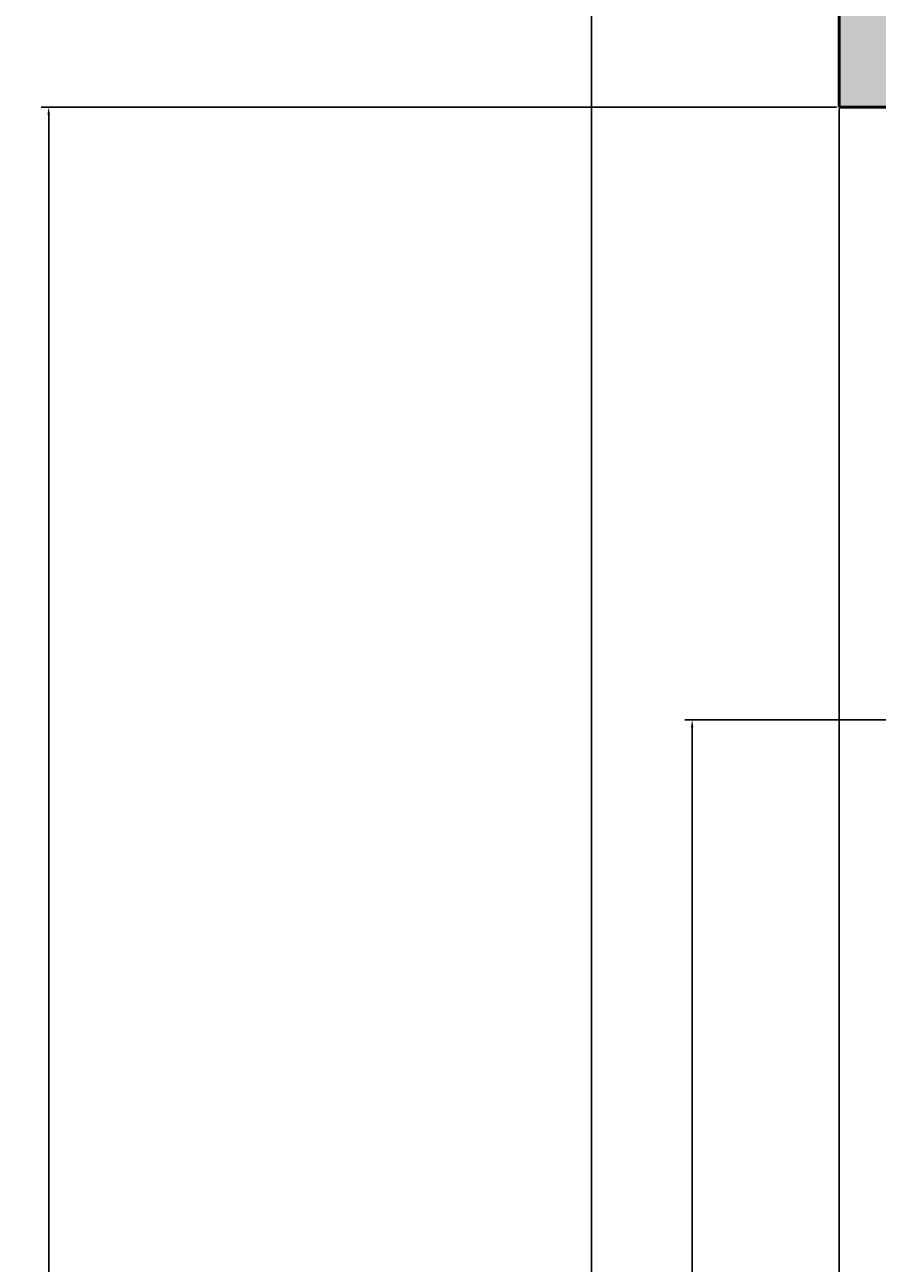
# Model space of a CAD drawing. Units: inches. Extents: x 2307 to 2544, y 2171 to 2540.
# Tile 37 of 52: x 2472 to 2493, y 2407 to 2438. Entities that reach past the tile are written whole.
import ezdxf

# ---------------------------------------------------------------- set-up
doc = ezdxf.new("R2010")
doc.units = ezdxf.units.IN
for name, color, linetype, lineweight in [('A-ANNO-DIMS', 2, 'Continuous', 18), ('A-DOOR', 3, 'Continuous', 25), ('A-FLOR-CASE', 9, 'Continuous', 18), ('A-WALL', 7, 'Continuous', 50)]:
    doc.layers.add(name, color=color, linetype=linetype, lineweight=lineweight)
doc.layers.add('A-WALL-PATT', color=18, linetype='Continuous', lineweight=13, true_color=0x000000)
doc.styles.get("Standard").update_dxf_attribs({"font": 'arial.ttf'})
doc.dimstyles.get("Standard").update_dxf_attribs({"dimtxt": 0.18, "dimasz": 0.18, "dimexe": 0.18, "dimexo": 0.0625, "dimgap": 0.09, "dimtad": 0, "dimtih": 1, "dimtoh": 1, "dimdec": 4, "dimzin": 0, "dimdsep": 46, "dimtxsty": 'Standard', "dimcen": 0.09, "dimadec": 0, "dimazin": 0, "dimtfac": 1, "dimtdec": 4, "dimtofl": 0, "dimtmove": 0, "dimatfit": 3, "dimfxl": 1, "dimtolj": 1, "dimtzin": 0, "dimarcsym": 0})

# ---------------------------------------------------------------- blocks, each defined once
blk = doc.blocks.new('*U13')
blk.add_line((40, 0), (40, -6))
blk = doc.blocks.new('*D32')
at = {"layer": 'A-ANNO-DIMS', "color": 0, "lineweight": -2, "transparency": 16777216}
for p, q in [((2493.473, 2420.657), (2487.956, 2420.657)), ((2488.136, 2420.477), (2488.136, 2402.84)), ((2488.136, 2384.837), (2488.136, 2402.474)), ((2493.473, 2384.657), (2487.956, 2384.657))]:
    blk.add_line(p, q, dxfattribs=at)
at = {"layer": 'A-ANNO-DIMS', "color": 0, "transparency": 16777216}
for points in [[(2488.106, 2420.477), (2488.166, 2420.477), (2488.136, 2420.657)], [(2488.106, 2384.837), (2488.166, 2384.837), (2488.136, 2384.657)]]:
    blk.add_solid(points, dxfattribs=at)
at = {"layer": 'Defpoints', "color": 0, "transparency": 16777216}
for p in [(2493.536, 2420.657), (2488.136, 2384.657), (2493.536, 2384.657)]:
    blk.add_point(p, dxfattribs=at)
at = {"layer": 'A-ANNO-DIMS', "color": 0, "transparency": 16777216, "insert": (2488.136, 2402.657), "char_height": 0.18, "attachment_point": 5}
blk.add_mtext('\\A1;DOUBLE SINK 36', dxfattribs=at)
blk = doc.blocks.new('*D49')
at = {"layer": 'A-ANNO-DIMS', "color": 0, "lineweight": -2, "transparency": 16777216}
for p, q in [((2491.633, 2435.51), (2472.366, 2435.51)), ((2472.546, 2435.33), (2472.546, 2389.691)), ((2472.546, 2343.69), (2472.546, 2389.328)), ((2491.633, 2343.51), (2472.366, 2343.51))]:
    blk.add_line(p, q, dxfattribs=at)
at = {"layer": 'A-ANNO-DIMS', "color": 0, "transparency": 16777216}
for points in [[(2472.516, 2435.33), (2472.576, 2435.33), (2472.546, 2435.51)], [(2472.516, 2343.69), (2472.576, 2343.69), (2472.546, 2343.51)]]:
    blk.add_solid(points, dxfattribs=at)
at = {"layer": 'Defpoints', "color": 0, "transparency": 16777216}
for p in [(2472.546, 2435.51), (2491.696, 2435.51), (2491.696, 2343.51)]:
    blk.add_point(p, dxfattribs=at)
at = {"layer": 'A-ANNO-DIMS', "color": 0, "transparency": 16777216, "insert": (2472.546, 2389.51), "char_height": 0.18, "attachment_point": 5}
blk.add_mtext('\\A1;92', dxfattribs=at)
blk = doc.blocks.new('*D54')
at = {"layer": 'A-ANNO-DIMS', "color": 0, "lineweight": -2, "transparency": 16777216}
for p, q in [((2461.696, 2435.447), (2461.696, 2171.18)), ((2491.696, 2435.447), (2491.696, 2171.18)), ((2461.876, 2171.36), (2476.477, 2171.36)), ((2491.516, 2171.36), (2476.914, 2171.36))]:
    blk.add_line(p, q, dxfattribs=at)
at = {"layer": 'A-ANNO-DIMS', "color": 0, "transparency": 16777216}
for points in [[(2461.876, 2171.39), (2461.876, 2171.33), (2461.696, 2171.36)], [(2491.516, 2171.39), (2491.516, 2171.33), (2491.696, 2171.36)]]:
    blk.add_solid(points, dxfattribs=at)
at = {"layer": 'Defpoints', "color": 0, "transparency": 16777216}
for p in [(2461.696, 2435.51), (2491.696, 2435.51), (2491.696, 2171.36)]:
    blk.add_point(p, dxfattribs=at)
at = {"layer": 'A-ANNO-DIMS', "color": 0, "transparency": 16777216, "insert": (2476.696, 2171.36), "char_height": 0.18, "attachment_point": 5}
blk.add_mtext('\\A1;30', dxfattribs=at)
blk = doc.blocks.new('*D59')
at = {"layer": 'A-ANNO-DIMS', "color": 0, "lineweight": -2, "transparency": 16777216}
for p, q in [((2455.696, 2315.572), (2455.696, 2540.345)), ((2455.876, 2540.165), (2470.477, 2540.165)), ((2485.516, 2540.165), (2470.914, 2540.165)), ((2485.696, 2315.572), (2485.696, 2540.345))]:
    blk.add_line(p, q, dxfattribs=at)
at = {"layer": 'A-ANNO-DIMS', "color": 0, "transparency": 16777216}
for points in [[(2455.876, 2540.195), (2455.876, 2540.135), (2455.696, 2540.165)], [(2485.516, 2540.195), (2485.516, 2540.135), (2485.696, 2540.165)]]:
    blk.add_solid(points, dxfattribs=at)
at = {"layer": 'Defpoints', "color": 0, "transparency": 16777216}
for p in [(2455.696, 2540.165), (2455.696, 2315.51), (2485.696, 2315.51)]:
    blk.add_point(p, dxfattribs=at)
at = {"layer": 'A-ANNO-DIMS', "color": 0, "transparency": 16777216, "insert": (2470.696, 2540.165), "char_height": 0.18, "attachment_point": 5}
blk.add_mtext('\\A1;30', dxfattribs=at)
blk = doc.blocks.new('*D61')
at = {"layer": 'A-ANNO-DIMS', "color": 0, "lineweight": -2, "transparency": 16777216}
for p, q in [((2491.696, 2435.572), (2491.696, 2540.345)), ((2491.876, 2540.165), (2503.476, 2540.165)), ((2515.516, 2540.165), (2503.916, 2540.165)), ((2515.696, 2435.572), (2515.696, 2540.345))]:
    blk.add_line(p, q, dxfattribs=at)
at = {"layer": 'A-ANNO-DIMS', "color": 0, "transparency": 16777216}
for points in [[(2491.876, 2540.195), (2491.876, 2540.135), (2491.696, 2540.165)], [(2515.516, 2540.195), (2515.516, 2540.135), (2515.696, 2540.165)]]:
    blk.add_solid(points, dxfattribs=at)
at = {"layer": 'Defpoints', "color": 0, "transparency": 16777216}
for p in [(2515.696, 2540.165), (2491.696, 2435.51), (2515.696, 2435.51)]:
    blk.add_point(p, dxfattribs=at)
at = {"layer": 'A-ANNO-DIMS', "color": 0, "transparency": 16777216, "insert": (2503.696, 2540.165), "char_height": 0.18, "attachment_point": 5}
blk.add_mtext('\\A1;24', dxfattribs=at)

msp = doc.modelspace()

# ---------------------------------------------------------------- hatches: boundary and pattern name
at = {"layer": 'A-WALL-PATT'}
h = msp.add_hatch(color=256, dxfattribs=at)
h.dxf.hatch_style = 1
h.paths.add_polyline_path([(2433.6935, 2199.5096), (2415.6423, 2199.5096), (2415.6423, 2190.5096), (2433.7832, 2190.5096)], flags=17)
h.paths.add_polyline_path([(2367.6423, 2199.5096), (2335.6958, 2199.5096), (2335.6958, 2307.3983), (2326.6958, 2307.3983), (2326.6958, 2190.5096), (2367.6423, 2190.5096)])
h.paths.add_polyline_path([(2524.6958, 2520.5096), (2496.7832, 2520.5096), (2496.7832, 2515.5149), (2472.7832, 2515.5149), (2472.7832, 2520.5096), (2415.4028, 2520.5096), (2415.4028, 2511.5096), (2451.6958, 2511.5096), (2451.6958, 2439.5096), (2451.6958, 2391.5096), (2445.6958, 2391.5096), (2445.6958, 2387.5096), (2455.6958, 2387.5096), (2455.6958, 2435.5096), (2461.6958, 2435.5096), (2461.6958, 2439.5096), (2455.6958, 2439.5096), (2455.6958, 2511.5096), (2515.6958, 2511.5096), (2515.6958, 2439.5096), (2491.6958, 2439.5096), (2491.6958, 2435.5096), (2515.6958, 2435.5096), (2515.6958, 2319.5096), (2451.6958, 2319.5096), (2451.6958, 2281.5096), (2481.6958, 2281.5096), (2481.6958, 2225.5096), (2485.6958, 2225.5096), (2485.6958, 2285.5096), (2455.6958, 2285.5096), (2455.6958, 2315.5096), (2515.6958, 2315.5096), (2515.6958, 2199.5096), (2469.6952, 2199.5096), (2469.785, 2190.5096), (2524.6958, 2190.5096)])

# ---------------------------------------------------------------- linework, layer by layer
at = {"layer": 'A-FLOR-CASE'}
msp.add_line((2491.6958, 2435.5096), (2491.6958, 2343.5096), dxfattribs=at)
at = {"layer": 'A-WALL'}
for p, q in [((2491.6958, 2439.5096), (2491.6958, 2435.5096)), ((2491.6958, 2435.5096), (2515.6958, 2435.5096))]:
    msp.add_line(p, q, dxfattribs=at)

# ---------------------------------------------------------------- block references
at = {"layer": 'A-DOOR', "xscale": 0.75, "yscale": 0.75, "zscale": 0.75}
msp.add_blockref('*U13', (2461.6958, 2440.0096), dxfattribs=at)

# ---------------------------------------------------------------- dimensions: what is measured, and where the dimension line sits
at = {"layer": 'A-ANNO-DIMS'}
for base, p1, p2, picture, middle in [((2455.6958, 2540.1649), (2485.6958, 2315.5096), (2455.6958, 2315.5096), '*D59', (2470.6958, 2540.1649)), ((2515.6958, 2540.1649), (2491.6958, 2435.5096), (2515.6958, 2435.5096), '*D61', (2503.6958, 2540.1649)), ((2491.6958, 2171.3596), (2461.6958, 2435.5096), (2491.6958, 2435.5096), '*D54', (2476.6958, 2171.3596))]:
    dim = msp.add_linear_dim(base=base, p1=p1, p2=p2, dimstyle='Standard', override={"dimdec": 0, "dimlfac": 1, "dimrnd": 0, "dimzin": 0, "dimdsep": 46, "dimlunit": 2}, dxfattribs=at)
    dim.commit()
    dim.dimension.update_dxf_attribs({"geometry": picture, "text_midpoint": middle})
dim = msp.add_linear_dim(base=(2472.5458, 2435.5096), p1=(2491.6958, 2343.5096), p2=(2491.6958, 2435.5096), angle=90, dimstyle='Standard', override={"dimdec": 0, "dimlfac": 1, "dimrnd": 0, "dimzin": 0, "dimdsep": 46, "dimlunit": 2}, dxfattribs=at)
dim.commit()
dim.dimension.update_dxf_attribs({"geometry": '*D49', "text_midpoint": (2472.5458, 2389.5096)})
dim = msp.add_linear_dim(base=(2488.1356, 2384.6573), p1=(2493.5356, 2420.6573), p2=(2493.5356, 2384.6573), angle=270, text='DOUBLE SINK <>', dimstyle='Standard', override={"dimdec": 0, "dimlfac": 1, "dimrnd": 0, "dimzin": 0, "dimdsep": 46, "dimlunit": 2}, dxfattribs=at)
dim.commit()
dim.dimension.update_dxf_attribs({"geometry": '*D32', "text_midpoint": (2488.1356, 2402.6573)})

doc.saveas('drawing.dxf')
